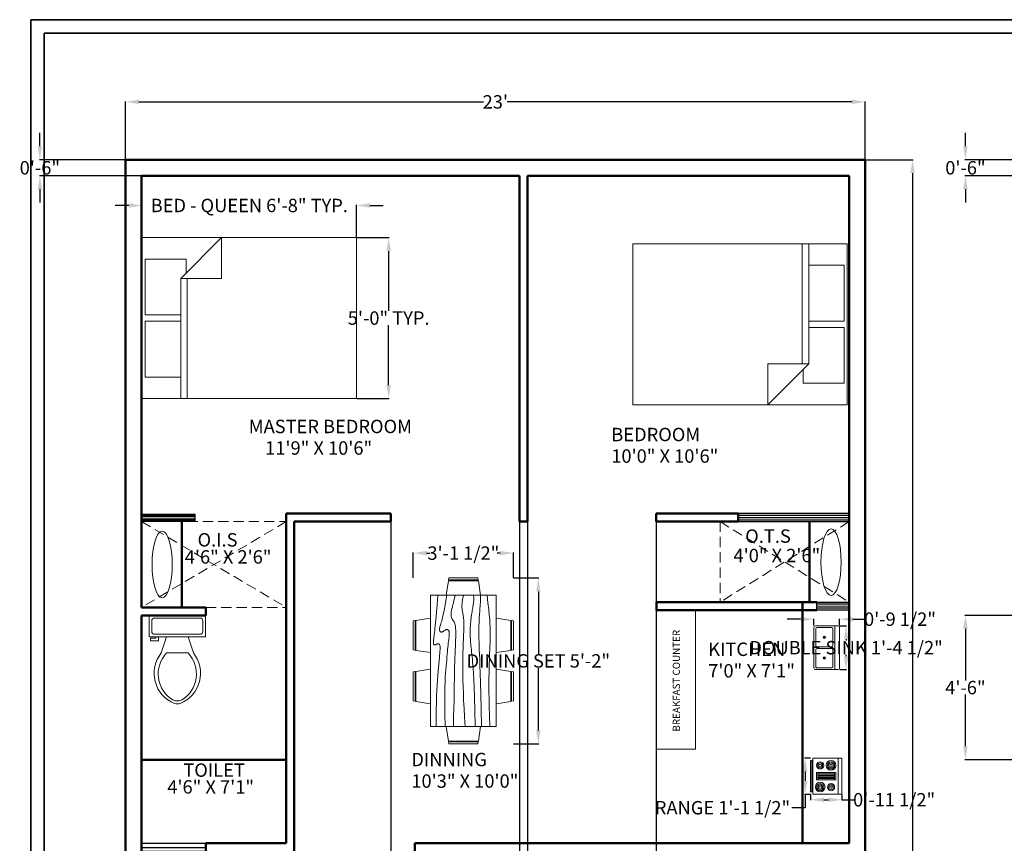
# Model space of a CAD drawing. Units: inches. Extents: x 396 to 1141, y -378 to 313.
# Tile 2 of 3: x 396 to 764, y 6 to 313. Entities that reach past the tile are written whole.
import ezdxf

# ---------------------------------------------------------------- set-up
doc = ezdxf.new("R2010")
doc.units = ezdxf.units.IN
doc.header["$MEASUREMENT"] = 0
doc.linetypes.add('DASHED', pattern=[19.05, 12.7, -6.35])
for name, color, linetype, lineweight in [('A-ANNO-DIMS', 2, 'Continuous', 18), ('A-ANNO-TTLB', 7, 'Continuous', 35), ('A-AREA-IDEN', 3, 'Continuous', 25), ('A-FLOR-FIXT', 150, 'Continuous', 18), ('A-FLOR-OVHD', 8, 'DASHED', 18), ('A-FURN', 30, 'Continuous', 18), ('A-GLAZ', 4, 'Continuous', 25), ('A-WALL', 7, 'Continuous', 50)]:
    doc.layers.add(name, color=color, linetype=linetype, lineweight=lineweight)
doc.styles.get("Standard").update_dxf_attribs({"font": 'arial.ttf'})
doc.dimstyles.get("Standard").update_dxf_attribs({"dimtxt": 5, "dimasz": 5, "dimexe": 0.18, "dimexo": 0.0625, "dimgap": 0.09, "dimtad": 0, "dimtih": 1, "dimtoh": 1, "dimdec": 1, "dimzin": 0, "dimdsep": 46, "dimlunit": 4, "dimtxsty": 'Standard', "dimcen": 0.09, "dimadec": 0, "dimazin": 0, "dimtfac": 1, "dimtdec": 1, "dimtofl": 0, "dimtmove": 0, "dimatfit": 3, "dimfxl": 1, "dimtolj": 1, "dimtzin": 0, "dimarcsym": 0})

# ---------------------------------------------------------------- blocks, each defined once
blk = doc.blocks.new('Dining Set - 36 x 72 in.')
for p, q in [((-22, 27.5), (-22.1562, 26.50042)), ((-22, 27.5), (-6, 27.5)), ((-5.8437, 26.49966), (-6, 27.5)), ((6, 27.5), (5.8438, 26.50042)), ((6, 27.5), (22, 27.5)), ((22.1563, 26.49966), (22, 27.5)), ((-22.2343, 26.00059), (-23.4847, 17.99762)), ((-22.2304, 26), (-5.7608, 26)), ((-5.8416, 26.5), (-22.1534, 26.5)), ((-4.5152, 17.99762), (-5.7655, 25.99926)), ((5.7657, 26.00059), (4.5153, 17.99762)), ((5.7696, 26), (22.2392, 26)), ((22.1584, 26.5), (5.8466, 26.5)), ((23.4848, 17.99762), (22.2345, 25.99926)), ((36, 18), (-36, 18)), ((-36, 18), (-36, -18)), ((36, -18), (36, 18)), ((-45.5, 8), (-44.5004, 8.15617)), ((-45.5, 8), (-45.5, -8)), ((-44.5, -8.15843), (-44.5, 8.15338)), ((-44.0006, 8.23428), (-35.9976, 9.48474)), ((-44, 8.23041), (-44, -8.23915)), ((44.0006, 8.23428), (35.9976, 9.48474)), ((44, 8.23041), (44, -8.23915)), ((44.5, -8.15843), (44.5, 8.15338)), ((45.5, 8), (44.5005, 8.15617)), ((45.5, 8), (45.5, -8)), ((-44.4997, -8.15631), (-45.5, -8)), ((-35.9976, -9.48476), (-43.9993, -8.2345)), ((35.9976, -9.48476), (43.9993, -8.2345)), ((44.4997, -8.15631), (45.5, -8)), ((-36, -18), (36, -18)), ((-22.2343, -26.0006), (-23.4847, -17.99762)), ((-4.5152, -17.99762), (-5.7655, -25.99928)), ((5.7657, -26.0006), (4.5153, -17.99762)), ((23.4848, -17.99762), (22.2345, -25.99928)), ((-22.2304, -26), (-5.7608, -26)), ((-22, -27.5), (-22.1562, -26.50044)), ((-5.8416, -26.5), (-22.1534, -26.5)), ((-5.8437, -26.49967), (-6, -27.5)), ((5.7696, -26), (22.2392, -26)), ((6, -27.5), (5.8438, -26.50044)), ((22.1584, -26.5), (5.8466, -26.5)), ((22.1563, -26.49967), (22, -27.5)), ((-22, -27.5), (-6, -27.5)), ((6, -27.5), (22, -27.5))]:
    blk.add_line(p, q)
for points in [[(-36, 15), (-31.1772, 14.97754), (-26.8079, 14.91406), (-22.8538, 14.81543), (-19.276, 14.6875), (-16.0362, 14.53613), (-13.0957, 14.36718), (-10.4159, 14.18652), (-7.9583, 14), (-5.6904, 13.81315), (-3.6035, 13.63021), (-1.6954, 13.45508), (0.0365, 13.29166), (1.5945, 13.14388), (2.9811, 13.01562), (4.1988, 12.9108), (5.25, 12.83333), (6.1393, 12.78613), (6.8802, 12.76823), (7.4883, 12.77767), (7.9792, 12.8125), (8.3685, 12.87077), (8.6719, 12.95052), (8.9049, 13.0498), (9.0833, 13.16666), (9.2205, 13.29899), (9.3216, 13.44401), (9.3895, 13.59879), (9.4271, 13.76041), (9.4373, 13.92594), (9.4232, 14.09245), (9.3875, 14.257), (9.3333, 14.41666), (9.2638, 14.56917), (9.1836, 14.71484), (9.0975, 14.85465), (9.0104, 14.98958), (8.9272, 15.1206), (8.8529, 15.2487), (8.7922, 15.37483), (8.75, 15.5), (8.7305, 15.62467), (8.7344, 15.74739), (8.7617, 15.86621), (8.8125, 15.97916), (8.8867, 16.08431), (8.9844, 16.17968), (9.1055, 16.26334), (9.25, 16.33333), (9.4189, 16.38802), (9.6172, 16.42708), (9.8506, 16.45052), (10.125, 16.45833), (10.4463, 16.45052), (10.8203, 16.42708), (11.2529, 16.38802), (11.75, 16.33333), (12.3184, 16.26318), (12.9694, 16.17838), (13.7151, 16.07991), (14.5677, 15.96875), (15.5395, 15.84586), (16.6426, 15.71224), (17.8893, 15.56884), (19.2917, 15.41666), (20.859, 15.25667), (22.5879, 15.08984), (24.4721, 14.91715), (26.5052, 14.73958), (28.6809, 14.5581), (30.9929, 14.3737), (33.4347, 14.18733), (36, 14)], [(-36, 10), (-28.9766, 10.14274), (-23.1725, 10.20442), (-18.4241, 10.19775), (-14.5677, 10.13541), (-11.4399, 10.03011), (-8.877, 9.89453), (-6.7154, 9.74137), (-4.7917, 9.58333), (-2.9698, 9.43082), (-1.2246, 9.28515), (0.4415, 9.14534), (2.026, 9.01041), (3.5266, 8.87939), (4.9408, 8.7513), (6.266, 8.62516), (7.5, 8.5), (8.6411, 8.37549), (9.6914, 8.2539), (10.6538, 8.13818), (11.5312, 8.03125), (12.3267, 7.93603), (13.043, 7.85547), (13.6831, 7.79248), (14.25, 7.75), (14.7471, 7.7303), (15.1797, 7.73307), (15.5537, 7.75732), (15.875, 7.80208), (16.1494, 7.86637), (16.3828, 7.94922), (16.5811, 8.04964), (16.75, 8.16666), (16.8944, 8.29915), (17.0143, 8.44531), (17.1089, 8.60319), (17.1771, 8.77083), (17.218, 8.94629), (17.2305, 9.1276), (17.2137, 9.31282), (17.1667, 9.5), (17.0895, 9.6875), (16.987, 9.875), (16.8649, 10.0625), (16.7292, 10.25), (16.5856, 10.4375), (16.4401, 10.625), (16.2985, 10.8125), (16.1667, 11), (16.05, 11.18733), (15.9518, 11.3737), (15.8752, 11.5581), (15.8229, 11.73958), (15.798, 11.91715), (15.8034, 12.08984), (15.842, 12.25667), (15.9167, 12.41666), (16.0295, 12.56836), (16.1784, 12.70833), (16.3605, 12.83268), (16.5729, 12.9375), (16.8127, 13.01888), (17.0768, 13.07291), (17.3625, 13.0957), (17.6667, 13.08333), (17.9894, 13.03312), (18.3418, 12.94726), (18.7382, 12.82918), (19.1927, 12.68229), (19.7195, 12.51001), (20.3327, 12.31575), (21.0465, 12.10294), (21.875, 11.875), (22.8357, 11.63354), (23.959, 11.37304), (25.2786, 11.08618), (26.8282, 10.76562), (28.6414, 10.40405), (30.752, 9.99414), (33.1936, 9.52856), (36, 9)], [(-36, 5.5), (-30.7157, 5.3348), (-26.069, 5.20963), (-21.9946, 5.11767), (-18.4271, 5.05208), (-15.3009, 5.00602), (-12.5508, 4.97265), (-10.1112, 4.94515), (-7.9167, 4.91666), (-5.909, 4.88167), (-4.0586, 4.83984), (-2.3429, 4.79215), (-0.7396, 4.73958), (0.7739, 4.6831), (2.22, 4.6237), (3.6213, 4.56233), (5, 4.5), (6.373, 4.43782), (7.7344, 4.3776), (9.0723, 4.32129), (10.375, 4.27083), (11.6309, 4.22819), (12.8281, 4.19531), (13.9551, 4.17415), (15, 4.16666), (15.954, 4.17448), (16.819, 4.19791), (17.6001, 4.23698), (18.3021, 4.29166), (18.9299, 4.36198), (19.4883, 4.44791), (19.9823, 4.54948), (20.4167, 4.66666), (20.7969, 4.79899), (21.1302, 4.94401), (21.4245, 5.09879), (21.6875, 5.26041), (21.9271, 5.42594), (22.1511, 5.59245), (22.3672, 5.757), (22.5834, 5.91666), (22.8065, 6.06868), (23.0404, 6.21093), (23.2879, 6.34147), (23.5521, 6.45833), (23.8358, 6.55957), (24.142, 6.64323), (24.4735, 6.70735), (24.8334, 6.75), (25.2235, 6.76969), (25.642, 6.76692), (26.0858, 6.74267), (26.5521, 6.69791), (27.0379, 6.63362), (27.5404, 6.55078), (28.0565, 6.45036), (28.5834, 6.33333), (29.1242, 6.19987), (29.7071, 6.04687), (30.3661, 5.87044), (31.1354, 5.66666), (32.0493, 5.43164), (33.142, 5.16146), (34.4475, 4.85221), (36, 4.5)], [(-36, -1), (-30.7915, -0.6591), (-26.0195, -0.38216), (-21.6519, -0.16284), (-17.6563, 0.00521), (-14.0005, 0.12833), (-10.6523, 0.21289), (-7.5796, 0.26522), (-4.75, 0.29166), (-2.134, 0.29793), (0.2878, 0.28711), (2.5317, 0.26163), (4.6146, 0.22396), (6.5529, 0.17651), (8.3633, 0.12174), (10.0623, 0.06209), (11.6667, 0), (13.1899, -0.06201), (14.6341, -0.1211), (15.9982, -0.17432), (17.2813, -0.21875), (18.4823, -0.25147), (19.6003, -0.26953), (20.6343, -0.27002), (21.5834, -0.25), (22.4481, -0.20768), (23.2357, -0.14584), (23.9549, -0.06836), (24.6146, 0.02083), (25.2235, 0.11784), (25.7904, 0.21875), (26.3241, 0.31966), (26.8334, 0.41666), (27.3265, 0.50618), (27.8099, 0.58593), (28.2894, 0.65397), (28.7709, 0.70833), (29.2601, 0.74707), (29.763, 0.76823), (30.2855, 0.76985), (30.8334, 0.75), (31.4088, 0.70784), (31.9994, 0.64713), (32.589, 0.57275), (33.1615, 0.48958), (33.7008, 0.4025), (34.1908, 0.3164), (34.6153, 0.23616), (34.9584, 0.16666), (35.2099, 0.11165), (35.3848, 0.07031), (35.504, 0.04069), (35.5886, 0.02083), (35.6594, 0.00879), (35.7377, 0.0026), (35.8442, 0.00032), (36, 0)], [(-36, -6.5), (-27.1843, -6.31267), (-20.084, -6.1263), (-14.469, -5.9419), (-10.1094, -5.76042), (-6.7752, -5.58285), (-4.2363, -5.41016), (-2.2629, -5.24333), (-0.625, -5.08334), (0.8708, -4.93099), (2.2715, -4.78646), (3.5872, -4.64974), (4.8281, -4.52084), (6.0046, -4.39974), (7.127, -4.28646), (8.2053, -4.18099), (9.25, -4.08334), (10.2705, -3.99382), (11.2734, -3.91407), (12.2647, -3.84603), (13.25, -3.79167), (14.2354, -3.75293), (15.2266, -3.73177), (16.2295, -3.73015), (17.25, -3.75), (18.2912, -3.79248), (19.3451, -3.85547), (20.4009, -3.93604), (21.4479, -4.03125), (22.4754, -4.13819), (23.4727, -4.25391), (24.4289, -4.37549), (25.3334, -4.5), (26.1785, -4.62492), (26.9694, -4.74935), (27.7145, -4.87281), (28.4219, -4.99479), (29.1, -5.11483), (29.7572, -5.23242), (30.4016, -5.34709), (31.0417, -5.45834), (31.6837, -5.56437), (32.3262, -5.65821), (32.9658, -5.73153), (33.599, -5.77604), (34.2224, -5.78345), (34.8327, -5.74545), (35.4264, -5.65373), (36, -5.5)], [(-36, -10), (-26.4022, -9.81299), (-18.4675, -9.62891), (-11.9839, -9.45069), (-6.7396, -9.28125), (-2.5226, -9.12354), (0.8789, -8.98047), (3.6769, -8.85498), (6.0833, -8.75), (8.2767, -8.66765), (10.3021, -8.60677), (12.1712, -8.56543), (13.8958, -8.54167), (15.4876, -8.53353), (16.9583, -8.53907), (18.3197, -8.55632), (19.5834, -8.58334), (20.7616, -8.61841), (21.8685, -8.66081), (22.9188, -8.71004), (23.9271, -8.76563), (24.9081, -8.82707), (25.8763, -8.89388), (26.8465, -8.96558), (27.8334, -9.04167), (28.8474, -9.12118), (29.8828, -9.20117), (30.93, -9.27824), (31.9792, -9.34896), (33.0205, -9.40991), (34.0443, -9.45768), (35.0407, -9.48885), (36, -9.5)], [(-36, -14.5), (-30.0881, -14.33513), (-25.0332, -14.21224), (-20.7312, -14.12647), (-17.0781, -14.07292), (-13.97, -14.04671), (-11.3027, -14.04297), (-8.9724, -14.05681), (-6.875, -14.08334), (-4.9224, -14.11833), (-3.0905, -14.16016), (-1.3709, -14.20785), (0.2448, -14.26042), (1.7647, -14.3169), (3.1973, -14.3763), (4.5507, -14.43767), (5.8333, -14.5), (7.0554, -14.5621), (8.235, -14.62175), (9.3922, -14.67652), (10.5469, -14.72396), (11.7192, -14.76164), (12.929, -14.78711), (14.1965, -14.79794), (15.5417, -14.79167), (16.9933, -14.76424), (18.6152, -14.70508), (20.4804, -14.60197), (22.6615, -14.44271), (25.2312, -14.21509), (28.2624, -13.9069), (31.8277, -13.50594), (36, -13)]]:
    blk.add_lwpolyline(points)
blk = doc.blocks.new('Range-Oven - 30 in top')
for p, q in [((0, -3), (30, -3)), ((12, -6), (18, -6)), ((13, -20), (13, -6)), ((14, -6), (14, -20)), ((15, -20), (15, -6)), ((16, -6), (16, -20)), ((17, -20), (17, -6)), ((6, -24), (6, -25)), ((8, -25), (8, -24)), ((18, -20), (12, -20)), ((22, -25), (22, -24)), ((24, -24), (24, -25))]:
    blk.add_line(p, q)
for points in [[(0, -24), (0, 0), (30, 0), (30, -24)], [(12, -21), (12, -5), (18, -5), (18, -21)], [(2, -26), (2, -25), (28, -25), (28, -26)]]:
    blk.add_lwpolyline(points, close=True)
for centre, radius in [((6, -9), 4), ((6, -9), 3), ((6, -9), 2), ((6, -9), 1), ((24, -9), 3), ((24, -9), 2), ((24, -9), 1), ((6, -18), 3), ((6, -18), 2), ((24, -18), 4), ((24, -18), 3), ((24, -18), 2), ((6, -18), 1), ((24, -18), 1)]:
    blk.add_circle(centre, radius)
blk = doc.blocks.new('Sink-double - 36 in top')
for p, q in [((-18, -4), (18, -4)), ((-0.75, -18.5), (-0.75, -6.5)), ((0.75, -6.5), (0.75, -18.5))]:
    blk.add_line(p, q)
for points in [[(-16.5, 0), (16.5, 0)], [(-18, -19.5), (-18, -1.5)], [(-16.5, -18.5), (-16.5, -6.5)], [(-15.5, -5.5), (-1.75, -5.5)], [(1.75, -5.5), (15.5, -5.5)], [(16.5, -6.5), (16.5, -18.5)], [(18, -1.5), (18, -19.5)], [(16.5, -21), (-16.5, -21)], [(-1.75, -19.5), (-15.5, -19.5)], [(15.5, -19.5), (1.75, -19.5)]]:
    blk.add_lwpolyline(points)
for centre, radius in [((-8.5, -12.5), 1), ((-8.5, -12.5), 0.5), ((8.5, -12.5), 1), ((8.5, -12.5), 0.5)]:
    blk.add_circle(centre, radius)
for centre, radius, start, end in [((-16.5, -1.5), 1.5, 90, 180), ((16.5, -1.5), 1.5, 0, 90), ((-15.5, -6.5), 1, 90, 180), ((-1.75, -6.5), 1, 0, 90), ((1.75, -6.5), 1, 90, 180), ((15.5, -6.5), 1, 0, 90), ((-16.5, -19.5), 1.5, 180, 270), ((-15.5, -18.5), 1, 180, 270), ((-1.75, -18.5), 1, 270, 0), ((1.75, -18.5), 1, 180, 270), ((15.5, -18.5), 1, 270, 0), ((16.5, -19.5), 1.5, 270, 0)]:
    blk.add_arc(centre, radius, start, end)
blk = doc.blocks.new('Bed - Queen')
for p, q in [((0, -80.00003), (0, 0)), ((0, 0), (59.99999, 0)), ((59.99999, 0), (59.99999, -80.00003)), ((7.99999, -1.2), (28.79998, -1.2)), ((7.99999, -14.4), (7.99999, -1.2)), ((28.79998, -1.2), (28.79998, -14.4)), ((31.19999, -1.2), (51.99999, -1.2)), ((31.19999, -14.4), (31.19999, -1.2)), ((51.99999, -1.2), (51.99999, -16.4)), ((0, -14.4), (44.8, -14.4)), ((59.99999, -29.6), (44.8, -14.4)), ((44.8, -14.4), (44.8, -29.6)), ((44.8, -16.8), (0, -16.8)), ((51.99999, -16.4), (46.79936, -16.4)), ((44.8, -29.6), (59.99999, -29.6)), ((59.99999, -80.00003), (0, -80.00003))]:
    blk.add_line(p, q)
blk = doc.blocks.new('*U6')
for p, q in [((9.5, -6), (9.5, -2)), ((-10, -8.5), (-8, -8.5)), ((-10, -9.5), (-10, -8.5)), ((-7, -9.5), (-10, -9.5)), ((-8, -8.5), (-8, -8)), ((-7, -8), (-7, -9.5)), ((-4, -8), (-6, -14)), ((4, -8), (6, -14)), ((4, -14), (-4, -14))]:
    blk.add_line(p, q)
blk.add_lwpolyline([(10.5, -8), (10.5, 0), (-10.5, 0), (-10.5, -8)], close=True)
for points in [[(-9.5, -2), (-9.5, -6)], [(8.5, -1), (-8.5, -1)], [(-8.5, -7), (8.5, -7)]]:
    blk.add_lwpolyline(points)
for centre, radius, start, end in [((-8.62, -1.88), 0.884, 81.8699, 188.1301), ((8.62, -1.88), 0.884, 351.8699, 98.1301), ((-8.62, -6.12), 0.884, 171.8699, 278.1301), ((8.62, -6.12), 0.884, 261.8699, 8.1301), ((3.52, -21.58), 12.17, 141.4691, 247.9714), ((4.2, -21.82), 11.33, 136.3677, 238.9468), ((-3.52, -21.58), 12.17, 292.0284, 38.5307), ((-4.2, -21.82), 11.33, 301.053, 43.6321), ((0, -27.88), 4, 245.7318, 294.2682), ((0, -29), 4, 254.8605, 285.1395)]:
    blk.add_arc(centre, radius, start, end)
blk = doc.blocks.new('*D9')
at = {"layer": 'A-ANNO-DIMS', "color": 0, "lineweight": -2, "ltscale": 0.3, "transparency": 16777216}
for p, q in [((435.61, 261.02), (435.61, 282.71)), ((440.61, 282.53), (569.24, 282.53)), ((706.61, 282.53), (577.99, 282.53)), ((711.61, 261.02), (711.61, 282.71))]:
    blk.add_line(p, q, dxfattribs=at)
at = {"layer": 'A-ANNO-DIMS', "color": 0, "ltscale": 0.3, "transparency": 16777216}
for points in [[(440.61, 283.37), (440.61, 281.7), (435.61, 282.53)], [(706.61, 283.37), (706.61, 281.7), (711.61, 282.53)]]:
    blk.add_solid(points, dxfattribs=at)
at = {"layer": 'Defpoints', "color": 0, "ltscale": 0.3, "transparency": 16777216}
for p in [(711.61, 282.53), (435.61, 260.95), (711.61, 260.95)]:
    blk.add_point(p, dxfattribs=at)
at = {"layer": 'A-ANNO-DIMS', "color": 0, "ltscale": 0.3, "transparency": 16777216, "insert": (573.61, 282.53), "char_height": 5, "attachment_point": 5}
blk.add_mtext("\\A1;23'", dxfattribs=at)
blk = doc.blocks.new('*D10')
at = {"layer": 'A-ANNO-DIMS', "color": 0, "lineweight": -2, "ltscale": 0.3, "transparency": 16777216}
for p, q in [((711.68, 260.95), (729.49, 260.95)), ((729.31, 255.95), (729.31, -31.9)), ((729.31, -325.05), (729.31, -37.19)), ((711.68, -330.05), (729.49, -330.05))]:
    blk.add_line(p, q, dxfattribs=at)
at = {"layer": 'A-ANNO-DIMS', "color": 0, "ltscale": 0.3, "transparency": 16777216}
for points in [[(728.47, 255.95), (730.14, 255.95), (729.31, 260.95)], [(728.47, -325.05), (730.14, -325.05), (729.31, -330.05)]]:
    blk.add_solid(points, dxfattribs=at)
at = {"layer": 'Defpoints', "color": 0, "ltscale": 0.3, "transparency": 16777216}
for p in [(711.61, 260.95), (711.61, -330.05), (729.31, -330.05)]:
    blk.add_point(p, dxfattribs=at)
at = {"layer": 'A-ANNO-DIMS', "color": 0, "ltscale": 0.3, "transparency": 16777216, "insert": (729.31, -34.55), "char_height": 5, "attachment_point": 5}
blk.add_mtext('\\A1;49\'-3"', dxfattribs=at)
blk = doc.blocks.new('WIN-1200')
at = {"ltscale": 0.3}
blk.add_line((664.23, 127.45), (705.61, 127.45), dxfattribs=at)
for points in [[(705.61, 128.95), (664.23, 128.95), (664.23, 125.95), (705.61, 125.95)], [(664.23, 128.38), (705.61, 128.38), (705.61, 126.44), (664.23, 126.44)]]:
    blk.add_lwpolyline(points, close=True, dxfattribs=at)
blk = doc.blocks.new('WIN-VENT-350')
at = {"ltscale": 0.3}
blk.add_line((693.61, 94.45), (705.61, 94.49), dxfattribs=at)
for points in [[(693.61, 95.95), (705.61, 95.95), (705.61, 92.95), (693.61, 92.95)], [(693.61, 95.26), (705.61, 95.26), (705.61, 93.72), (693.61, 93.72)]]:
    blk.add_lwpolyline(points, close=True, dxfattribs=at)
blk = doc.blocks.new('WIN-DUCT-700')
at = {"ltscale": 0.3}
blk.add_line((441.61, 4.45), (465.61, 4.45), dxfattribs=at)
blk.add_lwpolyline([(441.61, 5.95), (465.61, 5.95), (465.61, 2.95), (441.61, 2.95)], close=True, dxfattribs=at)
blk = doc.blocks.new('*D16')
at = {"layer": 'A-ANNO-DIMS', "color": 0, "lineweight": -2, "ltscale": 0.3, "transparency": 16777216}
for p, q in [((436.81, 243.89), (431.81, 243.89)), ((441.81, 231.95), (441.81, 244.07)), ((521.81, 231.95), (521.81, 244.07)), ((526.81, 243.89), (531.81, 243.89))]:
    blk.add_line(p, q, dxfattribs=at)
at = {"layer": 'A-ANNO-DIMS', "color": 0, "ltscale": 0.3, "transparency": 16777216}
for points in [[(436.81, 244.72), (436.81, 243.06), (441.81, 243.89)], [(526.81, 244.72), (526.81, 243.06), (521.81, 243.89)]]:
    blk.add_solid(points, dxfattribs=at)
at = {"layer": 'Defpoints', "color": 0, "ltscale": 0.3, "transparency": 16777216}
for p in [(441.81, 243.89), (441.81, 231.89), (521.81, 231.89)]:
    blk.add_point(p, dxfattribs=at)
at = {"layer": 'A-ANNO-DIMS', "color": 0, "ltscale": 0.3, "transparency": 16777216, "insert": (481.81, 243.89), "char_height": 5, "attachment_point": 5}
blk.add_mtext('\\A1;BED - QUEEN 6\'-8" TYP.', dxfattribs=at)
blk = doc.blocks.new('*D17')
at = {"layer": 'A-ANNO-DIMS', "color": 0, "lineweight": -2, "ltscale": 0.3, "transparency": 16777216}
for p, q in [((521.87, 231.89), (533.99, 231.89)), ((533.81, 226.89), (533.81, 204.53)), ((533.81, 176.89), (533.81, 199.25)), ((521.87, 171.89), (533.99, 171.89))]:
    blk.add_line(p, q, dxfattribs=at)
at = {"layer": 'A-ANNO-DIMS', "color": 0, "ltscale": 0.3, "transparency": 16777216}
for points in [[(532.98, 226.89), (534.64, 226.89), (533.81, 231.89)], [(532.98, 176.89), (534.64, 176.89), (533.81, 171.89)]]:
    blk.add_solid(points, dxfattribs=at)
at = {"layer": 'Defpoints', "color": 0, "ltscale": 0.3, "transparency": 16777216}
for p in [(521.81, 231.89), (533.81, 231.89), (521.81, 171.89)]:
    blk.add_point(p, dxfattribs=at)
at = {"layer": 'A-ANNO-DIMS', "color": 0, "ltscale": 0.3, "transparency": 16777216, "insert": (533.81, 201.89), "char_height": 5, "attachment_point": 5}
blk.add_mtext('\\A1;5\'-0" TYP.', dxfattribs=at)
blk = doc.blocks.new('*D24')
at = {"layer": 'A-ANNO-DIMS', "color": 0, "lineweight": -2, "ltscale": 0.3, "transparency": 16777216}
for p, q in [((580.44, 104.93), (589.84, 104.93)), ((589.66, 99.93), (589.66, 76.68)), ((589.66, 48.07), (589.66, 71.33)), ((580.44, 43.07), (589.84, 43.07))]:
    blk.add_line(p, q, dxfattribs=at)
at = {"layer": 'A-ANNO-DIMS', "color": 0, "ltscale": 0.3, "transparency": 16777216}
for points in [[(588.83, 99.93), (590.49, 99.93), (589.66, 104.93)], [(588.83, 48.07), (590.49, 48.07), (589.66, 43.07)]]:
    blk.add_solid(points, dxfattribs=at)
at = {"layer": 'Defpoints', "color": 0, "ltscale": 0.3, "transparency": 16777216}
for p in [(580.38, 104.93), (589.66, 104.93), (580.38, 43.07)]:
    blk.add_point(p, dxfattribs=at)
at = {"layer": 'A-ANNO-DIMS', "color": 0, "ltscale": 0.3, "transparency": 16777216, "insert": (589.66, 74), "char_height": 5, "attachment_point": 5}
blk.add_mtext('\\A1;DINING SET 5\'-2"', dxfattribs=at)
blk = doc.blocks.new('*D25')
at = {"layer": 'A-ANNO-DIMS', "color": 0, "lineweight": -2, "ltscale": 0.3, "transparency": 16777216}
for p, q in [((542.99, 105), (542.99, 114.39)), ((547.99, 114.21), (549.12, 114.21)), ((575.38, 114.21), (574.24, 114.21)), ((580.38, 105), (580.38, 114.39))]:
    blk.add_line(p, q, dxfattribs=at)
at = {"layer": 'A-ANNO-DIMS', "color": 0, "ltscale": 0.3, "transparency": 16777216}
for points in [[(547.99, 115.05), (547.99, 113.38), (542.99, 114.21)], [(575.38, 115.05), (575.38, 113.38), (580.38, 114.21)]]:
    blk.add_solid(points, dxfattribs=at)
at = {"layer": 'Defpoints', "color": 0, "ltscale": 0.3, "transparency": 16777216}
for p in [(542.99, 114.21), (542.99, 104.93), (580.38, 104.93)]:
    blk.add_point(p, dxfattribs=at)
at = {"layer": 'A-ANNO-DIMS', "color": 0, "ltscale": 0.3, "transparency": 16777216, "insert": (561.68, 114.21), "char_height": 5, "attachment_point": 5}
blk.add_mtext('\\A1;3\'-1 1/2"', dxfattribs=at)
blk = doc.blocks.new('*D26')
at = {"layer": 'A-ANNO-DIMS', "color": 0, "lineweight": -2, "ltscale": 0.3, "transparency": 16777216}
for p, q in [((691.17, 37.73), (689.02, 37.73)), ((689.2, 32.73), (689.2, 29.22)), ((691.17, 24.22), (689.02, 24.22)), ((689.2, 24.22), (689.2, 19.22)), ((689.2, 19.22), (684.2, 19.22))]:
    blk.add_line(p, q, dxfattribs=at)
at = {"layer": 'A-ANNO-DIMS', "color": 0, "ltscale": 0.3, "transparency": 16777216}
for points in [[(688.37, 32.73), (690.04, 32.73), (689.2, 37.73)], [(688.37, 29.22), (690.04, 29.22), (689.2, 24.22)]]:
    blk.add_solid(points, dxfattribs=at)
at = {"layer": 'Defpoints', "color": 0, "ltscale": 0.3, "transparency": 16777216}
for p in [(691.23, 37.73), (689.2, 24.22), (691.23, 24.22)]:
    blk.add_point(p, dxfattribs=at)
at = {"layer": 'A-ANNO-DIMS', "color": 0, "ltscale": 0.3, "transparency": 16777216, "insert": (658.38, 19.22), "char_height": 5, "attachment_point": 5}
blk.add_mtext('\\A1;RANGE 1\'-1 1/2"', dxfattribs=at)
blk = doc.blocks.new('*D27')
at = {"layer": 'A-ANNO-DIMS', "color": 0, "lineweight": -2, "ltscale": 0.3, "transparency": 16777216}
for p, q in [((691.23, 24.16), (691.23, 22.02)), ((696.23, 22.2), (697.93, 22.2)), ((702.93, 24.16), (702.93, 22.02)), ((702.93, 22.2), (707.93, 22.2))]:
    blk.add_line(p, q, dxfattribs=at)
at = {"layer": 'A-ANNO-DIMS', "color": 0, "ltscale": 0.3, "transparency": 16777216}
for points in [[(696.23, 23.03), (696.23, 21.37), (691.23, 22.2)], [(697.93, 23.03), (697.93, 21.37), (702.93, 22.2)]]:
    blk.add_solid(points, dxfattribs=at)
at = {"layer": 'Defpoints', "color": 0, "ltscale": 0.3, "transparency": 16777216}
for p in [(691.23, 24.22), (702.93, 24.22), (702.93, 22.2)]:
    blk.add_point(p, dxfattribs=at)
at = {"layer": 'A-ANNO-DIMS', "color": 0, "ltscale": 0.3, "transparency": 16777216, "insert": (722.43, 22.2), "char_height": 5, "attachment_point": 5}
blk.add_mtext('\\A1;0\'-11 1/2"', dxfattribs=at)
blk = doc.blocks.new('*D28')
at = {"layer": 'A-ANNO-DIMS', "color": 0, "lineweight": -2, "ltscale": 0.3, "transparency": 16777216}
for p, q in [((702.11, 87.1), (704.68, 87.1)), ((704.5, 82.1), (704.5, 81.61)), ((704.5, 75.75), (704.5, 76.25)), ((702.11, 70.75), (704.68, 70.75))]:
    blk.add_line(p, q, dxfattribs=at)
at = {"layer": 'A-ANNO-DIMS', "color": 0, "ltscale": 0.3, "transparency": 16777216}
for points in [[(703.67, 82.1), (705.33, 82.1), (704.5, 87.1)], [(703.67, 75.75), (705.33, 75.75), (704.5, 70.75)]]:
    blk.add_solid(points, dxfattribs=at)
at = {"layer": 'Defpoints', "color": 0, "ltscale": 0.3, "transparency": 16777216}
for p in [(702.05, 87.1), (702.05, 70.75), (704.5, 70.75)]:
    blk.add_point(p, dxfattribs=at)
at = {"layer": 'A-ANNO-DIMS', "color": 0, "ltscale": 0.3, "transparency": 16777216, "insert": (704.5, 78.93), "char_height": 5, "attachment_point": 5}
blk.add_mtext('\\A1;DOUBLE SINK 1\'-4 1/2"', dxfattribs=at)
blk = doc.blocks.new('*D29')
at = {"layer": 'A-ANNO-DIMS', "color": 0, "lineweight": -2, "ltscale": 0.3, "transparency": 16777216}
for p, q in [((687.51, 89.55), (682.51, 89.55)), ((692.51, 87.16), (692.51, 89.73)), ((702.05, 87.16), (702.05, 89.73)), ((707.05, 89.55), (712.05, 89.55))]:
    blk.add_line(p, q, dxfattribs=at)
at = {"layer": 'A-ANNO-DIMS', "color": 0, "ltscale": 0.3, "transparency": 16777216}
for points in [[(687.51, 90.39), (687.51, 88.72), (692.51, 89.55)], [(707.05, 90.39), (707.05, 88.72), (702.05, 89.55)]]:
    blk.add_solid(points, dxfattribs=at)
at = {"layer": 'Defpoints', "color": 0, "ltscale": 0.3, "transparency": 16777216}
for p in [(702.05, 89.55), (692.51, 87.1), (702.05, 87.1)]:
    blk.add_point(p, dxfattribs=at)
at = {"layer": 'A-ANNO-DIMS', "color": 0, "ltscale": 0.3, "transparency": 16777216, "insert": (724.61, 89.55), "char_height": 5, "attachment_point": 5}
blk.add_mtext('\\A1;0\'-9 1/2"', dxfattribs=at)
blk = doc.blocks.new('*D30')
at = {"layer": 'A-ANNO-DIMS', "color": 0, "lineweight": -2, "ltscale": 0.3, "transparency": 16777216}
for p, q in [((403.66, 265.95), (403.66, 270.95)), ((435.55, 260.95), (403.48, 260.95)), ((441.55, 254.95), (403.48, 254.95)), ((403.66, 249.95), (403.66, 244.95))]:
    blk.add_line(p, q, dxfattribs=at)
at = {"layer": 'A-ANNO-DIMS', "color": 0, "ltscale": 0.3, "transparency": 16777216}
for points in [[(402.83, 265.95), (404.5, 265.95), (403.66, 260.95)], [(402.83, 249.95), (404.5, 249.95), (403.66, 254.95)]]:
    blk.add_solid(points, dxfattribs=at)
at = {"layer": 'Defpoints', "color": 0, "ltscale": 0.3, "transparency": 16777216}
for p in [(435.61, 260.95), (403.66, 254.95), (441.61, 254.95)]:
    blk.add_point(p, dxfattribs=at)
at = {"layer": 'A-ANNO-DIMS', "color": 0, "ltscale": 0.3, "transparency": 16777216, "insert": (403.66, 257.95), "char_height": 5, "attachment_point": 5}
blk.add_mtext('\\A1;0\'-6"', dxfattribs=at)
blk = doc.blocks.new('*D32')
at = {"layer": 'A-ANNO-DIMS', "color": 0, "lineweight": -2, "ltscale": 0.3, "transparency": 16777216}
for p, q in [((582.61, 125.89), (582.61, -362.18)), ((585.61, 125.89), (585.61, -362.18)), ((577.61, -362), (572.61, -362)), ((590.61, -362), (595.61, -362))]:
    blk.add_line(p, q, dxfattribs=at)
at = {"layer": 'A-ANNO-DIMS', "color": 0, "ltscale": 0.3, "transparency": 16777216}
for points in [[(577.61, -361.16), (577.61, -362.83), (582.61, -362)], [(590.61, -361.16), (590.61, -362.83), (585.61, -362)]]:
    blk.add_solid(points, dxfattribs=at)
at = {"layer": 'Defpoints', "color": 0, "ltscale": 0.3, "transparency": 16777216}
for p in [(582.61, 125.95), (585.61, 125.95), (585.61, -362)]:
    blk.add_point(p, dxfattribs=at)
at = {"layer": 'A-ANNO-DIMS', "color": 0, "ltscale": 0.3, "transparency": 16777216, "insert": (602.35, -362), "char_height": 5, "attachment_point": 5}
blk.add_mtext('\\A1;0\'-3"', dxfattribs=at)
blk = doc.blocks.new('*D33')
at = {"layer": 'A-ANNO-DIMS', "color": 0, "lineweight": -2, "ltscale": 0.3, "transparency": 16777216}
for p, q in [((534.61, 125.89), (534.61, -362.18)), ((582.61, 125.89), (582.61, -362.18)), ((539.61, -362), (551.78, -362)), ((577.61, -362), (565.45, -362))]:
    blk.add_line(p, q, dxfattribs=at)
at = {"layer": 'A-ANNO-DIMS', "color": 0, "ltscale": 0.3, "transparency": 16777216}
for points in [[(539.61, -361.16), (539.61, -362.83), (534.61, -362)], [(577.61, -361.16), (577.61, -362.83), (582.61, -362)]]:
    blk.add_solid(points, dxfattribs=at)
at = {"layer": 'Defpoints', "color": 0, "ltscale": 0.3, "transparency": 16777216}
for p in [(534.61, 125.95), (582.61, 125.95), (582.61, -362)]:
    blk.add_point(p, dxfattribs=at)
at = {"layer": 'A-ANNO-DIMS', "color": 0, "ltscale": 0.3, "transparency": 16777216, "insert": (558.61, -362), "char_height": 5, "attachment_point": 5}
blk.add_mtext('\\A1;4\'-0"', dxfattribs=at)
blk = doc.blocks.new('*D34')
at = {"layer": 'A-ANNO-DIMS', "color": 0, "lineweight": -2, "ltscale": 0.3, "transparency": 16777216}
for p, q in [((585.61, 125.89), (585.61, -362.18)), ((633.61, 125.89), (633.61, -362.18)), ((590.61, -362), (602.78, -362)), ((628.61, -362), (616.45, -362))]:
    blk.add_line(p, q, dxfattribs=at)
at = {"layer": 'A-ANNO-DIMS', "color": 0, "ltscale": 0.3, "transparency": 16777216}
for points in [[(590.61, -361.16), (590.61, -362.83), (585.61, -362)], [(628.61, -361.16), (628.61, -362.83), (633.61, -362)]]:
    blk.add_solid(points, dxfattribs=at)
at = {"layer": 'Defpoints', "color": 0, "ltscale": 0.3, "transparency": 16777216}
for p in [(585.61, 125.95), (633.61, 125.95), (633.61, -362)]:
    blk.add_point(p, dxfattribs=at)
at = {"layer": 'A-ANNO-DIMS', "color": 0, "ltscale": 0.3, "transparency": 16777216, "insert": (609.61, -362), "char_height": 5, "attachment_point": 5}
blk.add_mtext('\\A1;4\'-0"', dxfattribs=at)
blk = doc.blocks.new('*D40')
at = {"layer": 'A-ANNO-DIMS', "color": 0, "lineweight": -2, "ltscale": 0.3, "transparency": 16777216}
for p, q in [((749.03, 265.95), (749.03, 270.95)), ((780.92, 260.95), (748.85, 260.95)), ((786.92, 254.95), (748.85, 254.95)), ((749.03, 249.95), (749.03, 244.95))]:
    blk.add_line(p, q, dxfattribs=at)
at = {"layer": 'A-ANNO-DIMS', "color": 0, "ltscale": 0.3, "transparency": 16777216}
for points in [[(748.2, 265.95), (749.87, 265.95), (749.03, 260.95)], [(748.2, 249.95), (749.87, 249.95), (749.03, 254.95)]]:
    blk.add_solid(points, dxfattribs=at)
at = {"layer": 'Defpoints', "color": 0, "ltscale": 0.3, "transparency": 16777216}
for p in [(780.98, 260.95), (749.03, 254.95), (786.98, 254.95)]:
    blk.add_point(p, dxfattribs=at)
at = {"layer": 'A-ANNO-DIMS', "color": 0, "ltscale": 0.3, "transparency": 16777216, "insert": (749.03, 257.95), "char_height": 5, "attachment_point": 5}
blk.add_mtext('\\A1;0\'-6"', dxfattribs=at)
blk = doc.blocks.new('*D45')
at = {"layer": 'A-ANNO-DIMS', "color": 0, "lineweight": -2, "ltscale": 0.3, "transparency": 16777216}
for p, q in [((840.92, 90.95), (748.85, 90.95)), ((749.03, 85.95), (749.03, 66.69)), ((749.03, 42.15), (749.03, 61.41)), ((840.92, 37.15), (748.85, 37.15))]:
    blk.add_line(p, q, dxfattribs=at)
at = {"layer": 'A-ANNO-DIMS', "color": 0, "ltscale": 0.3, "transparency": 16777216}
for points in [[(748.2, 85.95), (749.87, 85.95), (749.03, 90.95)], [(748.2, 42.15), (749.87, 42.15), (749.03, 37.15)]]:
    blk.add_solid(points, dxfattribs=at)
at = {"layer": 'Defpoints', "color": 0, "ltscale": 0.3, "transparency": 16777216}
for p in [(840.98, 90.95), (749.03, 37.15), (840.98, 37.15)]:
    blk.add_point(p, dxfattribs=at)
at = {"layer": 'A-ANNO-DIMS', "color": 0, "ltscale": 0.3, "transparency": 16777216, "insert": (749.03, 64.05), "char_height": 5, "attachment_point": 5}
blk.add_mtext('\\A1;4\'-6"', dxfattribs=at)

msp = doc.modelspace()

# ---------------------------------------------------------------- linework, layer by layer
at = {"layer": 'A-ANNO-TTLB', "ltscale": 0.3}
for points in [[(400.24, 313.19), (1105.01, 313.19), (1105.01, -377.62), (400.24, -377.62)], [(405.24, 308.19), (1100.01, 308.19), (1100.01, -372.62), (405.24, -372.62)]]:
    msp.add_lwpolyline(points, close=True, dxfattribs=at)
at = {"layer": 'A-FLOR-FIXT', "ltscale": 0.3}
for centre in [(449.3, 109.95), (698.89, 110.82)]:
    msp.add_ellipse(centre, major_axis=(0, -12.42), ratio=0.303469, dxfattribs=at)
at = {"layer": 'A-FLOR-OVHD', "ltscale": 0.3}
for p, q in [((441.61, 125.95), (495.61, 93.95)), ((495.61, 125.95), (441.61, 93.95)), ((441.61, 125.95), (495.61, 125.95)), ((657.56, 125.95), (657.56, 95.95)), ((657.56, 125.95), (705.61, 95.95)), ((705.61, 125.95), (657.56, 95.95)), ((465.61, 93.95), (495.61, 93.95))]:
    msp.add_line(p, q, dxfattribs=at)
at = {"layer": 'A-FURN', "ltscale": 0.3}
msp.add_lwpolyline([(633.71, 92.95), (648.31, 92.95), (648.31, 41.06), (633.71, 41.06)], close=True, dxfattribs=at)
at = {"layer": 'A-GLAZ', "ltscale": 0.3}
for points in [[(441.61, 128.69), (461.54, 128.69), (461.54, 125.95), (441.61, 125.95)], [(441.61, 128.23), (461.54, 128.23), (461.54, 126.43), (441.61, 126.43)], [(441.61, 127.82), (461.54, 127.82), (461.54, 126.9), (441.61, 126.9)]]:
    msp.add_lwpolyline(points, close=True, dxfattribs=at)
at = {"layer": 'A-WALL'}
for p, q in [((711.61, 260.95), (435.61, 260.95)), ((435.61, 260.95), (435.61, -330.05)), ((711.61, 260.95), (711.61, -330.05)), ((441.61, 254.95), (441.61, 125.95)), ((582.61, 254.95), (441.61, 254.95)), ((705.61, 254.95), (585.61, 254.95)), ((705.61, 254.95), (705.61, 5.95)), ((534.61, 128.95), (498.61, 128.95)), ((664.23, 128.95), (633.61, 128.95)), ((441.61, 125.95), (441.61, 93.95)), ((495.61, 125.95), (495.61, 5.95)), ((498.61, 125.95), (498.61, 2.95)), ((534.61, 125.95), (498.61, 125.95)), ((585.61, 125.95), (582.61, 125.95)), ((664.23, 125.95), (633.61, 125.95)), ((693.61, 95.95), (633.71, 95.95)), ((465.61, 93.95), (441.61, 93.95)), ((465.61, 93.95), (465.61, 90.95)), ((693.61, 92.95), (633.71, 92.95)), ((465.61, 90.95), (441.61, 90.95)), ((441.61, 90.95), (441.61, 5.95)), ((441.61, 5.95), (441.61, 2.95)), ((495.61, 5.95), (465.61, 5.95)), ((465.61, 2.95), (465.61, 5.95)), ((543.55, 5.95), (543.55, -39.05)), ((705.61, 5.95), (543.55, 5.95))]:
    msp.add_line(p, q, dxfattribs=at)
at = {"layer": 'A-WALL', "ltscale": 0.3}
for p, q in [((582.61, 125.95), (582.61, 254.95)), ((585.61, 125.95), (585.61, 254.95)), ((495.61, 125.95), (495.61, 128.95)), ((495.61, 128.95), (498.61, 128.95)), ((534.61, 128.95), (534.61, 125.95)), ((633.61, 128.95), (633.61, 125.95)), ((664.23, 128.95), (664.23, 125.95)), ((456.64, 125.95), (456.64, 93.95)), ((690.9, 125.95), (690.9, 95.95)), ((633.71, 95.95), (633.71, 92.95)), ((688.21, 95.95), (688.21, 5.95)), ((441.61, 37.15), (495.61, 37.15))]:
    msp.add_line(p, q, dxfattribs=at)

# ---------------------------------------------------------------- block references
at = {"layer": 'A-FLOR-FIXT', "ltscale": 0.3}
for name, p, xscale, yscale, zscale, rotation in [('Dining Set - 36 x 72 in.', (561.68, 74), 0.6798650627778576, 0.6798650627778576, 0.6798650627778576, 90), ('Sink-double - 36 in top', (702.05, 78.93), 0.4541063483313335, 0.4541063483313335, 0.4541063483313335, 270), ('Range-Oven - 30 in top', (702.93, 37.73), 0.4500465530572835, 0.4500465530572835, 0.4500465530572835, 270)]:
    msp.add_blockref(name, p, dxfattribs=dict(at, xscale=xscale, yscale=yscale, zscale=zscale, rotation=rotation))
at = {"layer": 'A-FLOR-FIXT'}
msp.add_blockref('*U6', (454.94, 90.95), dxfattribs=at)
at = {"layer": 'A-FURN', "ltscale": 0.3}
for p, rotation in [((441.81, 171.89), 90), ((704.94, 229.56), 270)]:
    msp.add_blockref('Bed - Queen', p, dxfattribs=dict(at, rotation=rotation))
at = {"layer": 'A-GLAZ'}
for name in ['WIN-1200', 'WIN-VENT-350', 'WIN-DUCT-700']:
    msp.add_blockref(name, (0, 0), dxfattribs=at)

# ---------------------------------------------------------------- texts
at = {"layer": 'A-AREA-IDEN', "ltscale": 0.3}
for s, p in [('MASTER BEDROOM', (481.61, 158.95)), ('BEDROOM', (616.88, 155.94)), ('    11\'9" X 10\'6"', (481.61, 150.91)), ('10\'0" X 10\'6"', (616.88, 147.91)), ('O.I.S', (462.5, 116.66)), ('O.T.S', (666.86, 118.05)), ('4\'6" X 2\'6"', (457.72, 110.29)), ('4\'0" X 2\'6"', (662.48, 110.81)), ('KITCHEN ', (653.05, 75.84)), ('7\'0" X 7\'1"', (653.05, 67.81)), ('DINNING', (542.27, 34.7)), ('TOILET', (457.19, 30.75)), ('4\'6" X 7\'1"', (451.21, 24.49)), ('10\'3" X 10\'0"', (542.27, 26.67))]:
    msp.add_text(s, height=5, dxfattribs=at).set_placement(p)
msp.add_text('BREAKFAST COUNTER', height=2.6841, rotation=90, dxfattribs=at).set_placement((642.5, 47.63))

# ---------------------------------------------------------------- dimensions: what is measured, and where the dimension line sits
at = {"layer": 'A-ANNO-DIMS', "ltscale": 0.3}
for base, p1, p2, override, picture, middle in [((711.61, 282.53), (435.61, 260.95), (711.61, 260.95), {"dimclrd": 0, "dimclre": 0, "dimclrt": 0}, '*D9', (573.61, 282.53)), ((582.61, -362), (534.61, 125.95), (582.61, 125.95), {"dimdec": 1, "dimlfac": 1, "dimrnd": 0, "dimzin": 1, "dimdsep": 46, "dimlunit": 4, "dimfrac": 2}, '*D33', (558.61, -362)), ((585.61, -362), (582.61, 125.95), (585.61, 125.95), {"dimdec": 1, "dimlfac": 1, "dimrnd": 0, "dimzin": 1, "dimdsep": 46, "dimlunit": 4, "dimfrac": 2}, '*D32', (602.35, -362)), ((633.61, -362), (585.61, 125.95), (633.61, 125.95), {"dimdec": 1, "dimlfac": 1, "dimrnd": 0, "dimzin": 1, "dimdsep": 46, "dimlunit": 4, "dimfrac": 2}, '*D34', (609.61, -362)), ((702.05, 89.55), (692.51, 87.1), (702.05, 87.1), {"dimdec": 1, "dimrnd": 0, "dimzin": 1, "dimlunit": 4, "dimfrac": 2}, '*D29', (724.61, 89.55)), ((702.93, 22.2), (691.23, 24.22), (702.93, 24.22), {"dimdec": 1, "dimrnd": 0, "dimzin": 1, "dimlunit": 4, "dimfrac": 2}, '*D27', (722.43, 22.2))]:
    dim = msp.add_linear_dim(base=base, p1=p1, p2=p2, dimstyle='Standard', override=override, dxfattribs=at)
    dim.commit()
    dim.dimension.update_dxf_attribs({"geometry": picture, "text_midpoint": middle})
for base, p1, p2, angle, override, picture, middle in [((403.66, 254.95), (435.61, 260.95), (441.61, 254.95), 90, {"dimdec": 1, "dimlfac": 1, "dimrnd": 0, "dimzin": 1, "dimdsep": 46, "dimlunit": 4, "dimfrac": 2}, '*D30', (403.66, 257.95)), ((749.03, 254.95), (780.98, 260.95), (786.98, 254.95), 90, {"dimdec": 1, "dimlfac": 1, "dimrnd": 0, "dimzin": 1, "dimdsep": 46, "dimlunit": 4, "dimfrac": 2}, '*D40', (749.03, 257.95)), ((729.31, -330.05), (711.61, 260.95), (711.61, -330.05), 90, {"dimclrd": 0, "dimclre": 0, "dimclrt": 0}, '*D10', (729.31, -34.55)), ((542.99, 114.21), (580.38, 104.93), (542.99, 104.93), 180, {"dimdec": 1, "dimrnd": 0, "dimzin": 1, "dimlunit": 4, "dimfrac": 2}, '*D25', (561.68, 114.21)), ((749.03, 37.15), (840.98, 90.95), (840.98, 37.15), 90, {"dimdec": 1, "dimlfac": 1, "dimrnd": 0, "dimzin": 1, "dimdsep": 46, "dimlunit": 4, "dimfrac": 2}, '*D45', (749.03, 64.05))]:
    dim = msp.add_linear_dim(base=base, p1=p1, p2=p2, angle=angle, dimstyle='Standard', override=override, dxfattribs=at)
    dim.commit()
    dim.dimension.update_dxf_attribs({"geometry": picture, "text_midpoint": middle})
for base, p1, p2, angle, text, picture, middle in [((441.81, 243.89), (521.81, 231.89), (441.81, 231.89), 180, 'BED - QUEEN <> TYP.', '*D16', (481.81, 243.89)), ((533.81, 231.89), (521.81, 171.89), (521.81, 231.89), 90, '<> TYP.', '*D17', (533.81, 201.89)), ((589.66, 104.93), (580.38, 43.07), (580.38, 104.93), 90, 'DINING SET <>', '*D24', (589.66, 74)), ((704.4985, 70.7543), (702.0464, 87.1021), (702.0464, 70.7543), 270, 'DOUBLE SINK <>', '*D28', (704.4985, 78.9282)), ((689.2, 24.22), (691.23, 37.73), (691.23, 24.22), 270, 'RANGE <>', '*D26', (658.38, 19.22))]:
    dim = msp.add_linear_dim(base=base, p1=p1, p2=p2, angle=angle, text=text, dimstyle='Standard', override={"dimdec": 1, "dimrnd": 0, "dimzin": 1, "dimlunit": 4, "dimfrac": 2}, dxfattribs=at)
    dim.commit()
    dim.dimension.update_dxf_attribs({"geometry": picture, "text_midpoint": middle})

doc.saveas('drawing.dxf')
